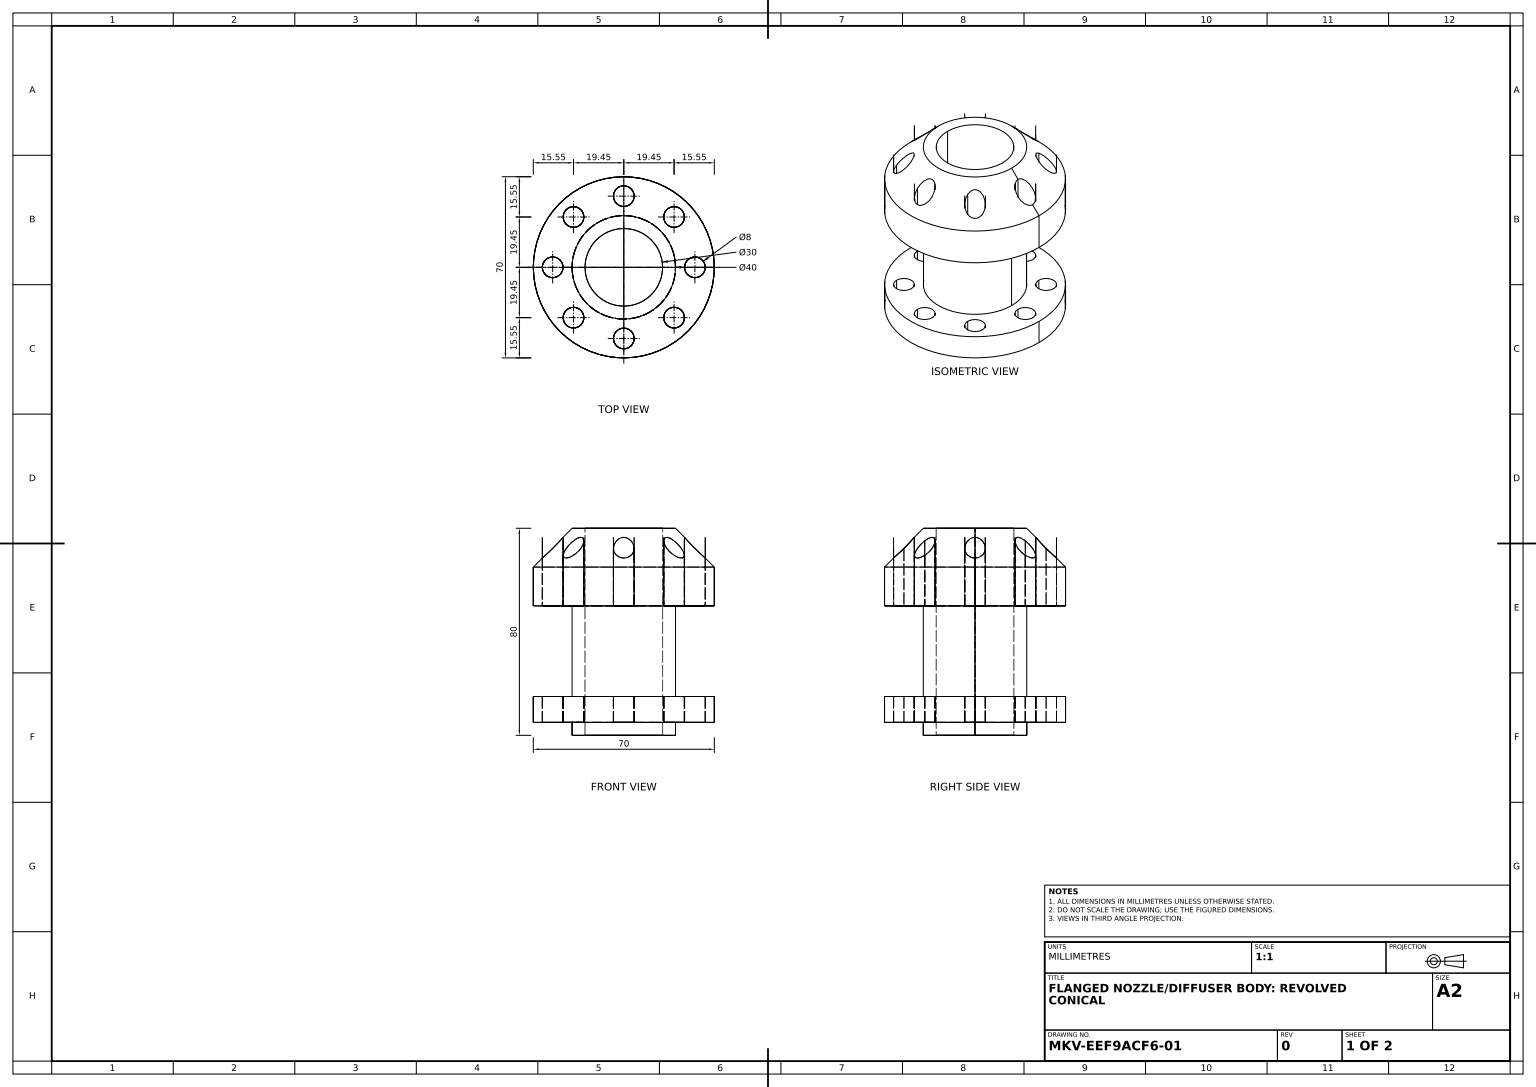
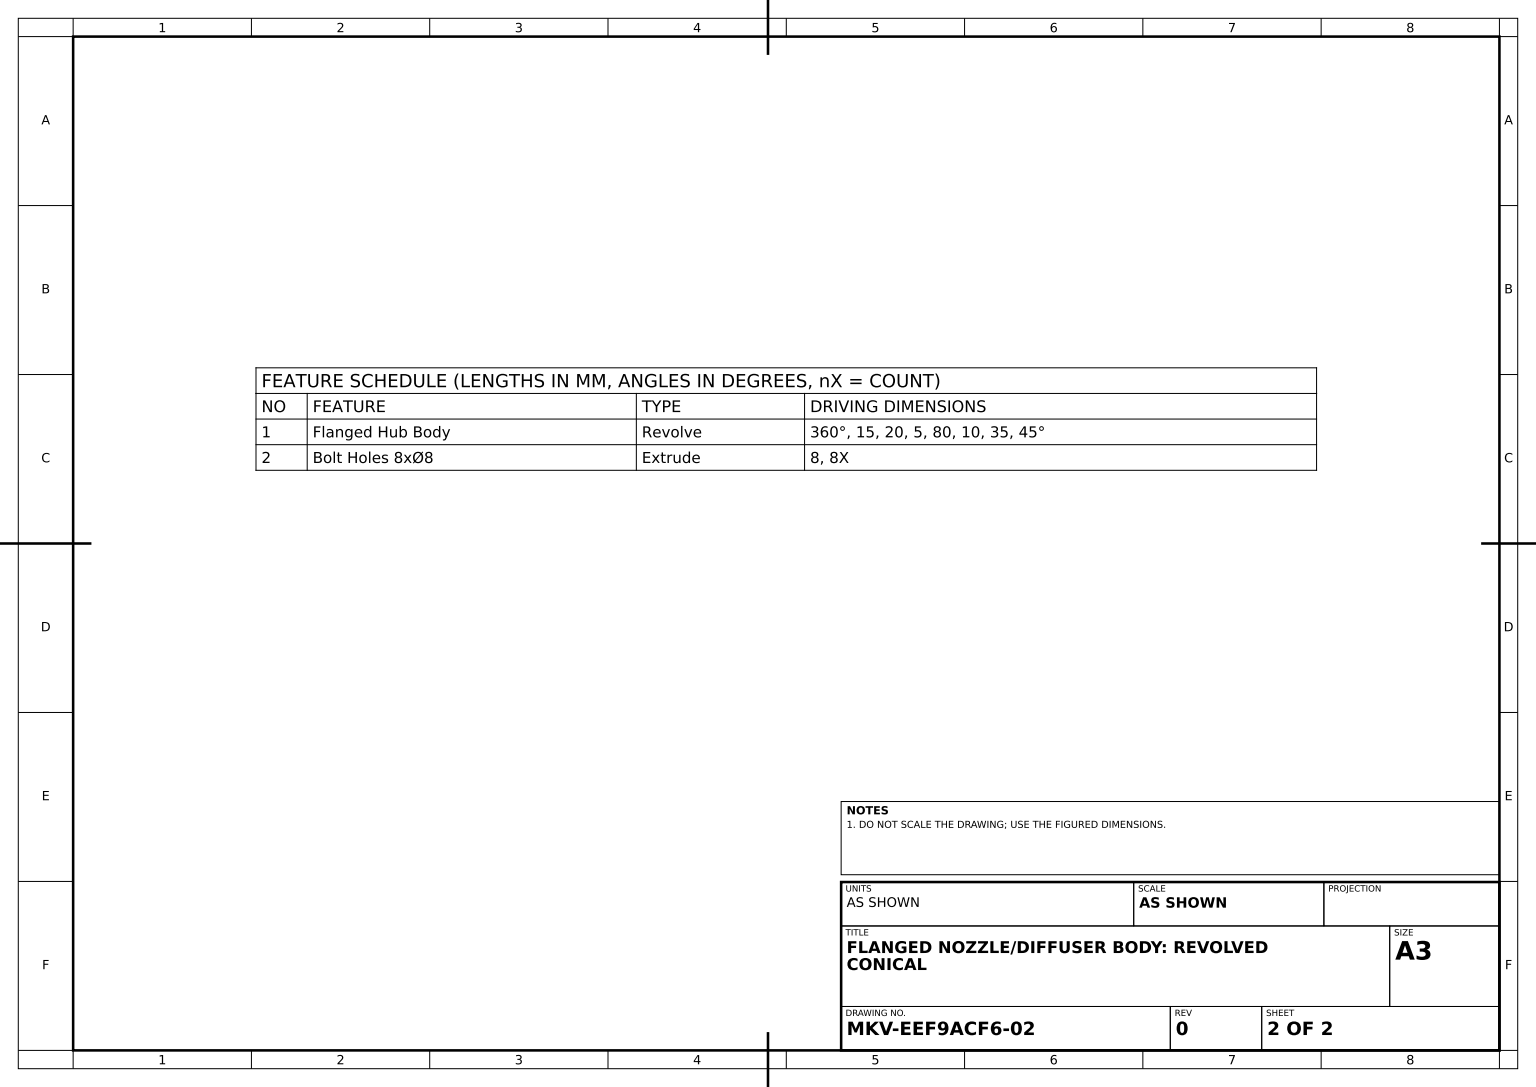
SolidWorks part; units mm, degrees
material "Plain Carbon Steel"
ref_plane "Front Plane" through (0, 0, 0) normal (0, 0, 1) x (1, 0, 0)
ref_plane "Top Plane" through (0, 0, 0) normal (0, 1, 0) x (1, 0, 0)
ref_plane "Right Plane" through (0, 0, 0) normal (1, 0, 0) x (0, 0, -1)
sketch "Hub Profile Sketch" plane through (0, 0, 0) normal (0, 0, 1) x (1, 0, 0)
  line L0 (0, 43.4605) -> (0, -40.7763) construction
  line L1 (-15, 40) -> (-15, -40)
  line L2 (-15, -40) -> (-20, -40)
  line L3 (-20, -40) -> (-20, -35)
  line L4 (-20, -35) -> (-35, -35)
  line L5 (-35, -35) -> (-35, -25)
  line L6 (-35, -25) -> (-20, -25)
  line L7 (-20, -25) -> (-20, 10)
  line L8 (-20, 10) -> (-35, 10)
  line L9 (-35, 10) -> (-35, 25)
  line L11 (-15, 40) -> (-20, 40)
  line L12 (-20, 40) -> (-35, 25)
  point P12 (-15, 0)
  dimension "D1" = 15
  dimension "D2" = 20
  dimension "D3" = 5
  dimension "D4" = 80
  dimension "D5" = 10
  dimension "D6" = 15
  dimension "D7" = 15
  dimension "D8" = 35
  dimension "D9" = 15
  dimension "D10" = 45
  dimension "D11" = 15
revolve "Flanged Hub Body" add sketch "Hub Profile Sketch" angle 360 about L0
sketch "Bolt Hole Circle Sketch" plane through (0, -35, 0) normal (0, -1, 0) x (1, 0, 0)
  circle A1 centre (27.5, 0) radius 4
  circle A2 centre (19.4454, -19.4454) radius 4
  circle A3 centre (0, -27.5) radius 4
  circle A4 centre (-19.4454, -19.4454) radius 4
  circle A5 centre (-27.5, 0) radius 4
  circle A6 centre (-19.4454, 19.4454) radius 4
  circle A7 centre (0, 27.5) radius 4
  circle A8 centre (19.4454, 19.4454) radius 4
  circle A9 centre (0, 0) radius 20 construction
  point P20 (0, 0)
  dimension "D1" = 8
  dimension "D2" = 19.4454
  dimension "D4" = 27.5
  dimension "D3" = 8
extrude "Bolt Holes 8xØ8" cut sketch "Bolt Hole Circle Sketch" against normal through all both and the other way through all
